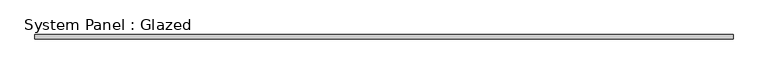
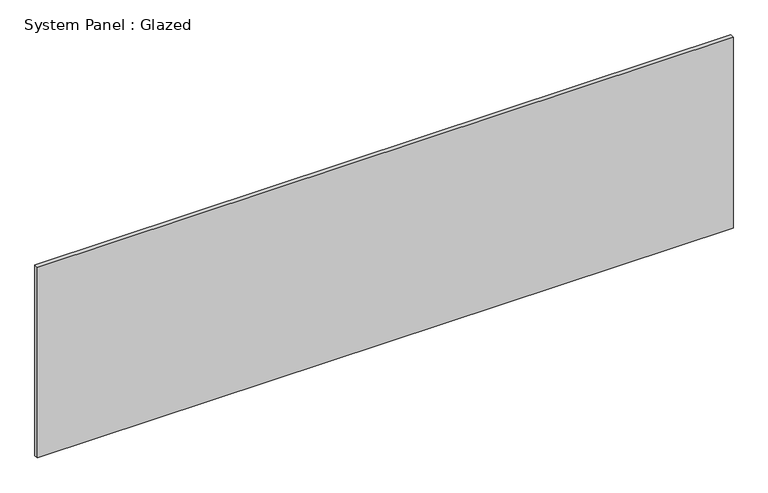
"""IFC4 building model written with IfcOpenShell, lengths in millimetres: plate geometry, System Panel : Glazed."""

from ifc_helpers import new_model, si_unit, origin, origin_with_axes, place, context, project, spatial, polyline, outline, extrude, source, transform, mapped, element, save


def system_panel_glazed_9c27a923(model_context):
    return source(origin(), model_context, "Body", "SweptSolid", [
        extrude(outline(polyline([(2108.2, 19.05), (-2108.2, 19.05), (-2108.2, 44.45), (2108.2, 44.45), (2108.2, 19.05)])), origin_with_axes(), (0.0, 0.0, 1.0), 1222.1336034),
    ])


if __name__ == "__main__":
    model = new_model("IFC4")
    model_context = context("Model", 3, world=origin())
    ifc_project = project(units=[si_unit("LENGTHUNIT", "METRE", prefix="MILLI")], contexts=[model_context])
    site = spatial("IfcSite", under=ifc_project)
    building = spatial("IfcBuilding", under=site)
    placement = place(None, origin())
    system_panel_glazed_shape = system_panel_glazed_9c27a923(model_context)
    element("IfcPlate", 1, ObjectType="System Panel : Glazed", at=placement, inside=building, context=model_context, shape_type="MappedRepresentation", body=[
        mapped(system_panel_glazed_shape, transform((0.0, 0.0, 0.0), x_axis=(1.0, 0.0, 0.0), y_axis=(0.0, 1.0, 0.0), z_axis=(0.0, 0.0, 1.0))),
    ])
    save(model, "model.ifc")

# Revit data of these elements
# Type "System Panel : Glazed"
#   Construction Type Id = "GSP4R"
#   Analytic Construction = "1/8 in Pilkington single glazing"
#   Visual Light Transmittance = 0.9
#   Solar Heat Gain Coefficient = 0.86
#   Heat Transfer Coefficient (U) = 1.18115 BTU/(h·ft²·°F)
#   Define Thermal Properties by = 1
# Element 1 (IfcPlate, "System Panel : Glazed")
#   Materials on its faces: "Glass"
# Materials
#   "Glass": class "Glass", colour RGB 0 128 192, transparency 0.75, Description = "Soda Lime Glass", Cost = 0
